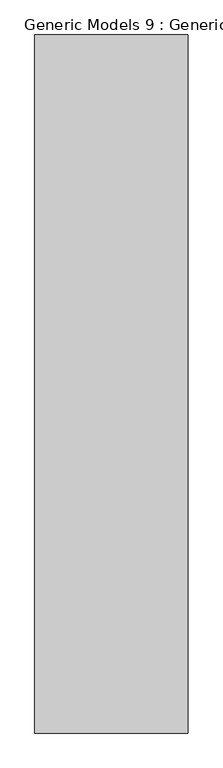
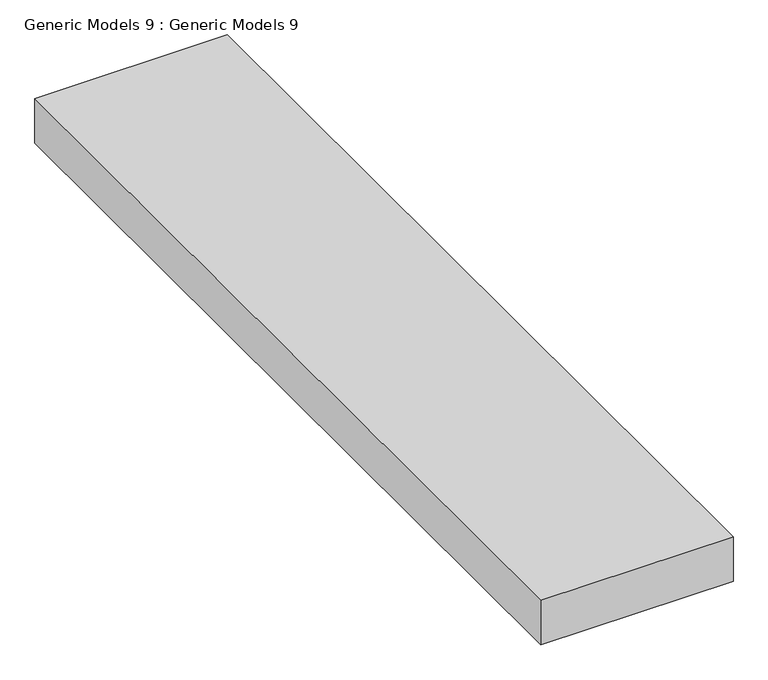
"""IFC4 building model written with IfcOpenShell, lengths in millimetres: proxy geometry, Generic Models 9 : Generic Models 9."""

from ifc_helpers import new_model, si_unit, frame, origin, place, context, project, spatial, polyline, outline, extrude, source, transform, mapped, element, save


def generic_models_9_generic_models_9_c0a8784b(model_context):
    return source(origin(), model_context, "Body", "SweptSolid", [
        extrude(outline(polyline([(-3177.6940223, -3914.3777232), (-3177.6940223, -6755.9095607), (-3802.4859258, -6755.9095607), (-3802.4859258, -3914.3777232), (-3177.6940223, -3914.3777232)])), frame((0.0, 0.0, 5410.2621354), z_axis=(0.0, 0.0, 1.0), x_axis=(1.0, 0.0, 0.0)), (0.0, 0.0, 1.0), 152.4),
    ])


if __name__ == "__main__":
    model = new_model("IFC4")
    model_context = context("Model", 3, world=origin())
    ifc_project = project(units=[si_unit("LENGTHUNIT", "METRE", prefix="MILLI")], contexts=[model_context])
    site = spatial("IfcSite", under=ifc_project)
    building = spatial("IfcBuilding", under=site)
    placement = place(None, origin())
    generic_models_9_generic_models_9_shape = generic_models_9_generic_models_9_c0a8784b(model_context)
    element("IfcBuildingElementProxy", 1, Name="Generic Models 9 : Generic Models 9", ObjectType="Generic Models 9 : Generic Models 9", at=placement, inside=building, context=model_context, shape_type="MappedRepresentation", body=[
        mapped(generic_models_9_generic_models_9_shape, transform((0.0, 0.0, 0.0), x_axis=(1.0, 0.0, 0.0), y_axis=(0.0, 1.0, 0.0), z_axis=(0.0, 0.0, 1.0))),
    ])
    save(model, "model.ifc")
